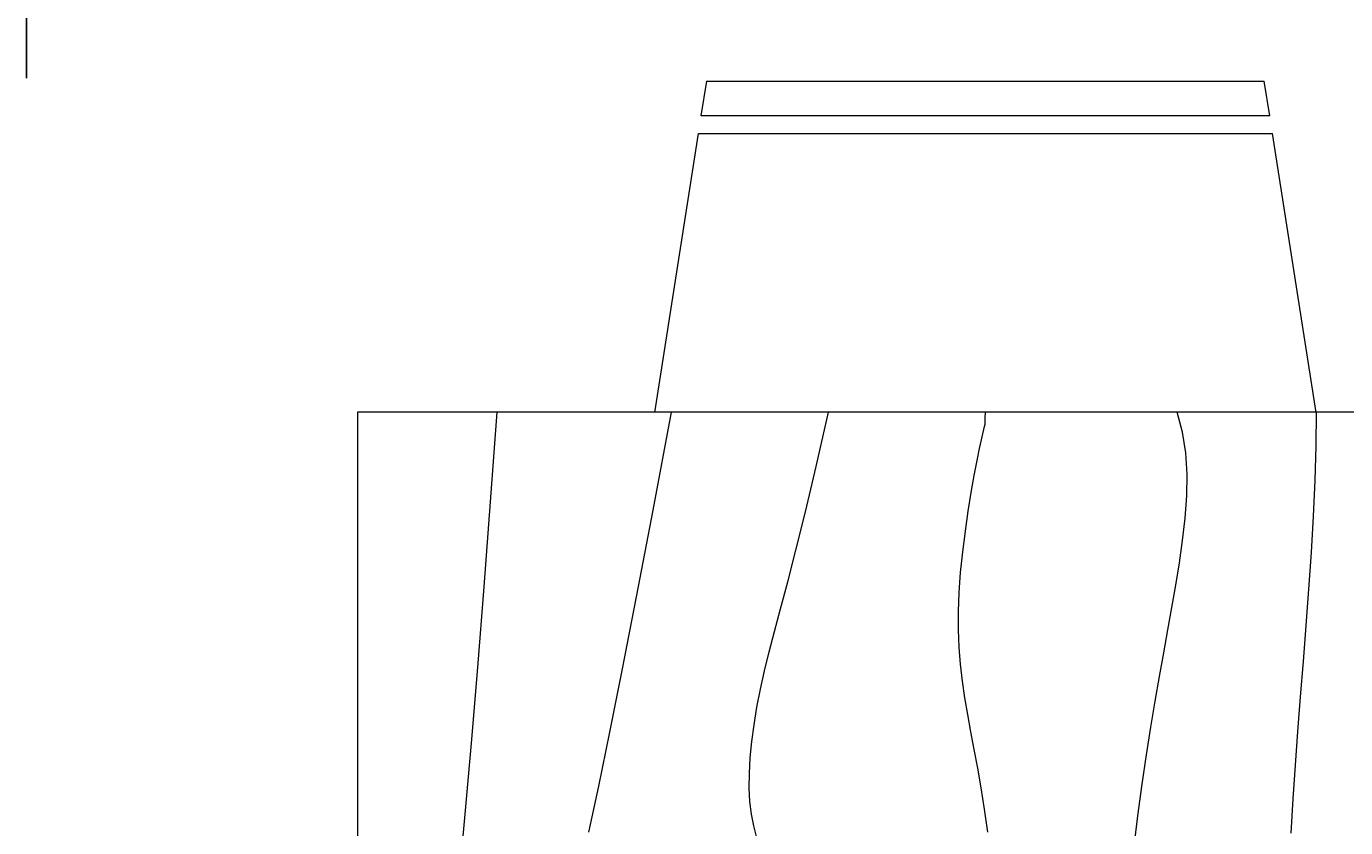
# Model space of a CAD drawing. Units: inches. Extents: x -301 to 715, y -607 to 364.
# Tile 111 of 141: x -41 to -12, y 175 to 192. Entities that reach past the tile are written whole.
import ezdxf

# ---------------------------------------------------------------- set-up
doc = ezdxf.new("R2010")
doc.units = ezdxf.units.IN
doc.header["$MEASUREMENT"] = 0
doc.layers.add('A-ANNO-DIMS', color=2, linetype='Continuous', lineweight=18)
doc.layers.add('A-FURN', color=8, linetype='Continuous', lineweight=18)
doc.styles.get("Standard").update_dxf_attribs({"font": 'arial.ttf'})
doc.dimstyles.get("Standard").update_dxf_attribs({"dimtxt": 0.18, "dimasz": 0.18, "dimexe": 0.18, "dimexo": 0.0625, "dimgap": 0.09, "dimtad": 0, "dimtih": 1, "dimtoh": 1, "dimdec": 1, "dimzin": 0, "dimdsep": 46, "dimlunit": 4, "dimtxsty": 'Standard', "dimcen": 0.09, "dimclrd": 3, "dimclre": 4, "dimclrt": 6, "dimadec": 0, "dimazin": 0, "dimtfac": 1, "dimtdec": 1, "dimtofl": 0, "dimtmove": 0, "dimatfit": 3, "dimfxl": 1, "dimtfill": 2, "dimtfillclr": 51, "dimtolj": 1, "dimtzin": 0, "dimarcsym": 0})

# ---------------------------------------------------------------- blocks, each defined once
blk = doc.blocks.new('Dining Set - 36 x 72 in.')
for p, q in [((36, 18), (-36, 18)), ((36, -18), (36, 18)), ((44.0006, 8.23428), (35.9976, 9.48474)), ((44, 8.23041), (44, -8.23915)), ((44.5, -8.15843), (44.5, 8.15338)), ((45.5, 8), (44.5005, 8.15617)), ((45.5, 8), (45.5, -8)), ((35.9976, -9.48476), (43.9993, -8.2345)), ((44.4997, -8.15631), (45.5, -8))]:
    blk.add_line(p, q)
for points in [[(22.5879, 15.08984), (24.4721, 14.91715), (26.5052, 14.73958), (28.6809, 14.5581), (30.9929, 14.3737), (33.4347, 14.18733), (36, 14)], [(23.959, 11.37304), (25.2786, 11.08618), (26.8282, 10.76562), (28.6414, 10.40405), (30.752, 9.99414), (33.1936, 9.52856), (36, 9)], [(23.8358, 6.55957), (24.142, 6.64323), (24.4735, 6.70735), (24.8334, 6.75), (25.2235, 6.76969), (25.642, 6.76692), (26.0858, 6.74267), (26.5521, 6.69791), (27.0379, 6.63362), (27.5404, 6.55078), (28.0565, 6.45036), (28.5834, 6.33333), (29.1242, 6.19987), (29.7071, 6.04687), (30.3661, 5.87044), (31.1354, 5.66666), (32.0493, 5.43164), (33.142, 5.16146), (34.4475, 4.85221), (36, 4.5)], [(23.9549, -0.06836), (24.6146, 0.02083), (25.2235, 0.11784), (25.7904, 0.21875), (26.3241, 0.31966), (26.8334, 0.41666), (27.3265, 0.50618), (27.8099, 0.58593), (28.2894, 0.65397), (28.7709, 0.70833), (29.2601, 0.74707), (29.763, 0.76823), (30.2855, 0.76985), (30.8334, 0.75), (31.4088, 0.70784), (31.9994, 0.64713), (32.589, 0.57275), (33.1615, 0.48958), (33.7008, 0.4025), (34.1908, 0.3164), (34.6153, 0.23616), (34.9584, 0.16666), (35.2099, 0.11165), (35.3848, 0.07031), (35.504, 0.04069), (35.5886, 0.02083), (35.6594, 0.00879), (35.7377, 0.0026), (35.8442, 0.00032), (36, 0)], [(23.4727, -4.25391), (24.4289, -4.37549), (25.3334, -4.5), (26.1785, -4.62492), (26.9694, -4.74935), (27.7145, -4.87281), (28.4219, -4.99479), (29.1, -5.11483), (29.7572, -5.23242), (30.4016, -5.34709), (31.0417, -5.45834), (31.6837, -5.56437), (32.3262, -5.65821), (32.9658, -5.73153), (33.599, -5.77604), (34.2224, -5.78345), (34.8327, -5.74545), (35.4264, -5.65373), (36, -5.5)], [(23.9271, -8.76563), (24.9081, -8.82707), (25.8763, -8.89388), (26.8465, -8.96558), (27.8334, -9.04167), (28.8474, -9.12118), (29.8828, -9.20117), (30.93, -9.27824), (31.9792, -9.34896), (33.0205, -9.40991), (34.0443, -9.45768), (35.0407, -9.48885), (36, -9.5)]]:
    blk.add_lwpolyline(points)
blk = doc.blocks.new('*D129')
at = {"layer": 'A-ANNO-DIMS', "color": 4, "lineweight": -2, "transparency": 16777216}
for p, q in [((-40.957, 191.37), (-40.957, 201.768)), ((0.469, 191.37), (0.469, 201.768))]:
    blk.add_line(p, q, dxfattribs=at)
at = {"layer": 'A-ANNO-DIMS', "color": 3, "lineweight": -2, "transparency": 16777216}
for p, q in [((-40.777, 201.588), (-20.783, 201.588)), ((0.289, 201.588), (-19.705, 201.588))]:
    blk.add_line(p, q, dxfattribs=at)
at = {"layer": 'A-ANNO-DIMS', "color": 3, "transparency": 16777216}
for points in [[(-40.777, 201.618), (-40.777, 201.558), (-40.957, 201.588)], [(0.289, 201.618), (0.289, 201.558), (0.469, 201.588)]]:
    blk.add_solid(points, dxfattribs=at)
at = {"layer": 'Defpoints', "color": 0, "transparency": 16777216}
for p in [(-40.957, 201.588), (-40.957, 191.307), (0.469, 191.307)]:
    blk.add_point(p, dxfattribs=at)
at = {"layer": 'A-ANNO-DIMS', "color": 6, "transparency": 16777216, "insert": (-20.244, 201.588), "char_height": 0.18, "attachment_point": 5, "bg_fill": 1, "box_fill_scale": 1.25, "bg_fill_color": 51, "bg_fill_transparency": 0}
blk.add_mtext('\\A1;3\'-5 1/2"', dxfattribs=at)

msp = doc.modelspace()

# ---------------------------------------------------------------- block references
at = {"layer": 'A-FURN', "xscale": 0.753207081168398, "yscale": 0.753207081168398, "zscale": 0.753207081168398, "rotation": 90}
msp.add_blockref('Dining Set - 36 x 72 in.', (-20.244, 157.036), dxfattribs=at)

# ---------------------------------------------------------------- dimensions: what is measured, and where the dimension line sits
at = {"layer": 'A-ANNO-DIMS'}
dim = msp.add_linear_dim(base=(-40.957, 201.588), p1=(0.469, 191.307), p2=(-40.957, 191.307), angle=180, dimstyle='Standard', override={"dimdec": 1, "dimlfac": 1, "dimrnd": 0, "dimzin": 1, "dimdsep": 46, "dimlunit": 4, "dimfrac": 2}, dxfattribs=at)
dim.commit()
dim.dimension.update_dxf_attribs({"geometry": '*D129', "text_midpoint": (-20.244, 201.588)})

doc.saveas('drawing.dxf')
